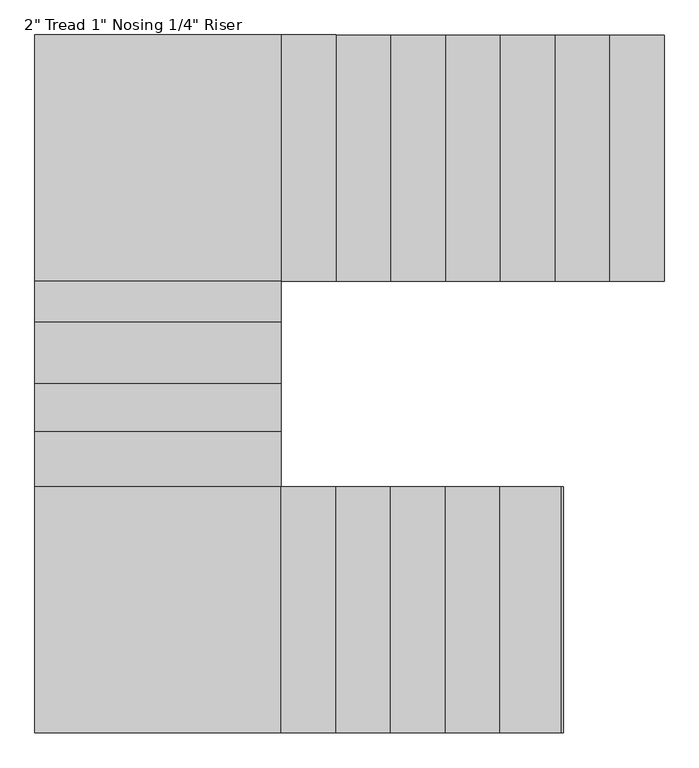
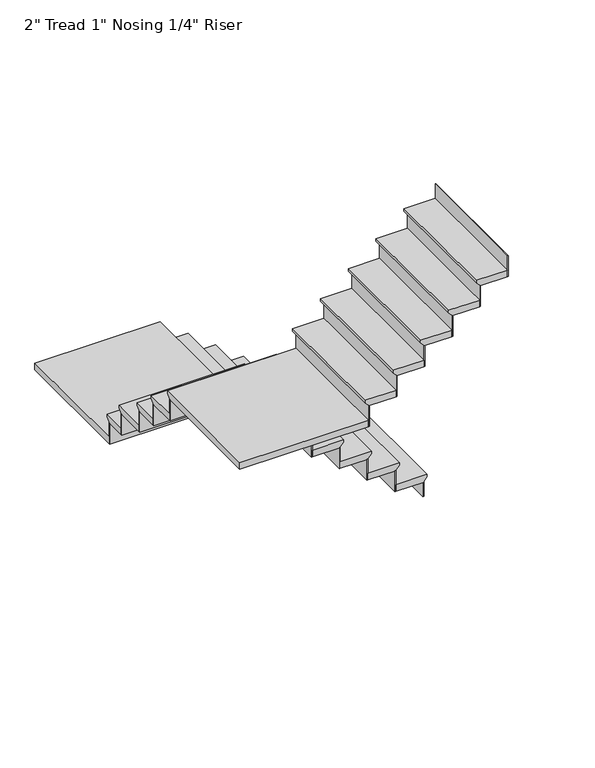
"""IFC4 building model written with IfcOpenShell, lengths in millimetres: stair flight geometry."""

from ifc_helpers import new_model, si_unit, origin, place, context, project, spatial, faceted_brep, source, transform, mapped, element, save


def stair_flight_03a67781(model_context):
    return source(origin(), model_context, "Body", "Brep", [
        faceted_brep([(-3603.1340247, 922.0319954, 9742.5710526), (-3603.1340247, 922.0319954, 9761.6210526), (-3603.1340247, 7.6319954, 9761.6210526), (-3603.1340247, 7.6319954, 9742.5710526), (-3628.5340247, 922.0319954, 9717.1710526), (-3628.5340247, 7.6319954, 9717.1710526), (-3831.7340247, 922.0319954, 9761.6210526), (-3831.7340247, 7.6319954, 9761.6210526), (-3628.5340247, 7.6319954, 9710.8210526), (-3831.7340247, 7.6319954, 9710.8210526), (-3831.7340247, 922.0319954, 9710.8210526), (-3628.5340247, 922.0319954, 9710.8210526)], [[[0, 1, 2, 3]], [[4, 0, 3, 5]], [[2, 1, 6, 7]], [[8, 9, 10, 11]], [[2, 7, 9, 8, 5, 3]], [[8, 11, 4, 5]], [[6, 1, 0, 4, 11, 10]], [[7, 6, 10, 9]]]),
        faceted_brep([(-3628.5340247, 922.0319954, 9710.8210526), (-3628.5340247, 922.0319954, 9601.2), (-3634.8840247, 922.0319954, 9601.2), (-3634.8840247, 922.0319954, 9710.8210526), (-3628.5340247, 7.6319954, 9710.8210526), (-3634.8840247, 7.6319954, 9710.8210526), (-3634.8840247, 7.6319954, 9601.2), (-3628.5340247, 7.6319954, 9601.2)], [[[0, 1, 2, 3]], [[4, 5, 6, 7]], [[1, 0, 4, 7]], [[2, 1, 7, 6]], [[3, 2, 6, 5]], [[0, 3, 5, 4]]]),
        faceted_brep([(-3831.7340247, 922.0319954, 9871.2421053), (-3831.7340247, 922.0319954, 9710.8210526), (-3838.0840247, 922.0319954, 9710.8210526), (-3838.0840247, 922.0319954, 9871.2421053), (-3831.7340247, 7.6319954, 9871.2421053), (-3838.0840247, 7.6319954, 9871.2421053), (-3838.0840247, 7.6319954, 9710.8210526), (-3831.7340247, 7.6319954, 9710.8210526)], [[[0, 1, 2, 3]], [[4, 5, 6, 7]], [[1, 0, 4, 7]], [[2, 1, 7, 6]], [[3, 2, 6, 5]], [[0, 3, 5, 4]]]),
        faceted_brep([(-3806.3340247, 7.6319954, 9922.0421053), (-3806.3340247, 922.0319954, 9922.0421053), (-4034.9340247, 922.0319954, 9922.0421053), (-4034.9340247, 7.6319954, 9922.0421053), (-3831.7340247, 7.6319954, 9871.2421053), (-4034.9340247, 7.6319954, 9871.2421053), (-4034.9340247, 922.0319954, 9871.2421053), (-3831.7340247, 922.0319954, 9871.2421053), (-3831.7340247, 7.6319954, 9877.5921053), (-3806.3340247, 7.6319954, 9902.9921053), (-3831.7340247, 922.0319954, 9877.5921053), (-3806.3340247, 922.0319954, 9902.9921053)], [[[0, 1, 2, 3]], [[4, 5, 6, 7]], [[0, 3, 5, 4, 8, 9]], [[4, 7, 10, 8]], [[2, 1, 11, 10, 7, 6]], [[3, 2, 6, 5]], [[11, 1, 0, 9]], [[10, 11, 9, 8]]]),
        faceted_brep([(-4034.9340247, 922.0319954, 10031.6631579), (-4034.9340247, 922.0319954, 9871.2421053), (-4041.2840247, 922.0319954, 9871.2421053), (-4041.2840247, 922.0319954, 10031.6631579), (-4034.9340247, 7.6319954, 10031.6631579), (-4041.2840247, 7.6319954, 10031.6631579), (-4041.2840247, 7.6319954, 9871.2421053), (-4034.9340247, 7.6319954, 9871.2421053)], [[[0, 1, 2, 3]], [[4, 5, 6, 7]], [[1, 0, 4, 7]], [[2, 1, 7, 6]], [[3, 2, 6, 5]], [[0, 3, 5, 4]]]),
        faceted_brep([(-4009.5340247, 7.6319954, 10082.4631579), (-4009.5340247, 922.0319954, 10082.4631579), (-4238.1340247, 922.0319954, 10082.4631579), (-4238.1340247, 7.6319954, 10082.4631579), (-4034.9340247, 7.6319954, 10031.6631579), (-4238.1340247, 7.6319954, 10031.6631579), (-4238.1340247, 922.0319954, 10031.6631579), (-4034.9340247, 922.0319954, 10031.6631579), (-4034.9340247, 7.6319954, 10038.0131579), (-4009.5340247, 7.6319954, 10063.4131579), (-4034.9340247, 922.0319954, 10038.0131579), (-4009.5340247, 922.0319954, 10063.4131579)], [[[0, 1, 2, 3]], [[4, 5, 6, 7]], [[0, 3, 5, 4, 8, 9]], [[4, 7, 10, 8]], [[2, 1, 11, 10, 7, 6]], [[3, 2, 6, 5]], [[11, 1, 0, 9]], [[10, 11, 9, 8]]]),
        faceted_brep([(-4238.1340247, 922.0319954, 10192.0842105), (-4238.1340247, 922.0319954, 10031.6631579), (-4244.4840247, 922.0319954, 10031.6631579), (-4244.4840247, 922.0319954, 10192.0842105), (-4238.1340247, 7.6319954, 10192.0842105), (-4244.4840247, 7.6319954, 10192.0842105), (-4244.4840247, 7.6319954, 10031.6631579), (-4238.1340247, 7.6319954, 10031.6631579)], [[[0, 1, 2, 3]], [[4, 5, 6, 7]], [[1, 0, 4, 7]], [[2, 1, 7, 6]], [[3, 2, 6, 5]], [[0, 3, 5, 4]]]),
        faceted_brep([(-4212.7340247, 7.6319954, 10242.8842105), (-4212.7340247, 922.0319954, 10242.8842105), (-4441.3340247, 922.0319954, 10242.8842105), (-4441.3340247, 7.6319954, 10242.8842105), (-4238.1340247, 7.6319954, 10192.0842105), (-4441.3340247, 7.6319954, 10192.0842105), (-4441.3340247, 922.0319954, 10192.0842105), (-4238.1340247, 922.0319954, 10192.0842105), (-4238.1340247, 7.6319954, 10198.4342105), (-4212.7340247, 7.6319954, 10223.8342105), (-4238.1340247, 922.0319954, 10198.4342105), (-4212.7340247, 922.0319954, 10223.8342105)], [[[0, 1, 2, 3]], [[4, 5, 6, 7]], [[0, 3, 5, 4, 8, 9]], [[4, 7, 10, 8]], [[2, 1, 11, 10, 7, 6]], [[3, 2, 6, 5]], [[11, 1, 0, 9]], [[10, 11, 9, 8]]]),
        faceted_brep([(-4441.3340247, 922.0319954, 10352.5052632), (-4441.3340247, 922.0319954, 10192.0842105), (-4447.6840247, 922.0319954, 10192.0842105), (-4447.6840247, 922.0319954, 10352.5052632), (-4441.3340247, 7.6319954, 10352.5052632), (-4447.6840247, 7.6319954, 10352.5052632), (-4447.6840247, 7.6319954, 10192.0842105), (-4441.3340247, 7.6319954, 10192.0842105)], [[[0, 1, 2, 3]], [[4, 5, 6, 7]], [[1, 0, 4, 7]], [[2, 1, 7, 6]], [[3, 2, 6, 5]], [[0, 3, 5, 4]]]),
        faceted_brep([(-4415.9340247, 7.6319954, 10403.3052632), (-4415.9340247, 922.0319954, 10403.3052632), (-4644.5340247, 922.0319954, 10403.3052632), (-4644.5340247, 7.6319954, 10403.3052632), (-4441.3340247, 7.6319954, 10352.5052632), (-4644.5340247, 7.6319954, 10352.5052632), (-4644.5340247, 922.0319954, 10352.5052632), (-4441.3340247, 922.0319954, 10352.5052632), (-4441.3340247, 7.6319954, 10358.8552632), (-4415.9340247, 7.6319954, 10384.2552632), (-4441.3340247, 922.0319954, 10358.8552632), (-4415.9340247, 922.0319954, 10384.2552632)], [[[0, 1, 2, 3]], [[4, 5, 6, 7]], [[0, 3, 5, 4, 8, 9]], [[4, 7, 10, 8]], [[2, 1, 11, 10, 7, 6]], [[3, 2, 6, 5]], [[11, 1, 0, 9]], [[10, 11, 9, 8]]]),
        faceted_brep([(-4644.5340247, 922.0319954, 10512.9263158), (-4644.5340247, 922.0319954, 10352.5052632), (-4650.8840247, 922.0319954, 10352.5052632), (-4650.8840247, 922.0319954, 10512.9263158), (-4644.5340247, 7.6319954, 10512.9263158), (-4650.8840247, 7.6319954, 10512.9263158), (-4650.8840247, 7.6319954, 10352.5052632), (-4644.5340247, 7.6319954, 10352.5052632)], [[[0, 1, 2, 3]], [[4, 5, 6, 7]], [[1, 0, 4, 7]], [[2, 1, 7, 6]], [[3, 2, 6, 5]], [[0, 3, 5, 4]]]),
        faceted_brep([(-4619.1340247, 7.6319954, 10563.7263158), (-4619.1340247, 922.0319954, 10563.7263158), (-4847.7340247, 922.0319954, 10563.7263158), (-4847.7340247, 7.6319954, 10563.7263158), (-4644.5340247, 7.6319954, 10512.9263158), (-4847.7340247, 7.6319954, 10512.9263158), (-4847.7340247, 922.0319954, 10512.9263158), (-4644.5340247, 922.0319954, 10512.9263158), (-4644.5340247, 7.6319954, 10519.2763158), (-4619.1340247, 7.6319954, 10544.6763158), (-4644.5340247, 922.0319954, 10519.2763158), (-4619.1340247, 922.0319954, 10544.6763158)], [[[0, 1, 2, 3]], [[4, 5, 6, 7]], [[0, 3, 5, 4, 8, 9]], [[4, 7, 10, 8]], [[2, 1, 11, 10, 7, 6]], [[3, 2, 6, 5]], [[11, 1, 0, 9]], [[10, 11, 9, 8]]]),
        faceted_brep([(-4847.7340247, 922.0319954, 10673.3473684), (-4847.7340247, 922.0319954, 10512.9263158), (-4854.0840247, 922.0319954, 10512.9263158), (-4854.0840247, 922.0319954, 10673.3473684), (-4847.7340247, 7.6319954, 10673.3473684), (-4854.0840247, 7.6319954, 10673.3473684), (-4854.0840247, 7.6319954, 10512.9263158), (-4847.7340247, 7.6319954, 10512.9263158)], [[[0, 1, 2, 3]], [[4, 5, 6, 7]], [[1, 0, 4, 7]], [[2, 1, 7, 6]], [[3, 2, 6, 5]], [[0, 3, 5, 4]]]),
        faceted_brep([(-4822.3340247, 7.6319954, 10724.1473684), (-4822.3340247, 922.0319954, 10724.1473684), (-5050.9340247, 922.0319954, 10724.1473684), (-5050.9340247, 7.6319954, 10724.1473684), (-4847.7340247, 7.6319954, 10673.3473684), (-5050.9340247, 7.6319954, 10673.3473684), (-5050.9340247, 922.0319954, 10673.3473684), (-4847.7340247, 922.0319954, 10673.3473684), (-4847.7340247, 7.6319954, 10679.6973684), (-4822.3340247, 7.6319954, 10705.0973684), (-4847.7340247, 922.0319954, 10679.6973684), (-4822.3340247, 922.0319954, 10705.0973684)], [[[0, 1, 2, 3]], [[4, 5, 6, 7]], [[0, 3, 5, 4, 8, 9]], [[4, 7, 10, 8]], [[2, 1, 11, 10, 7, 6]], [[3, 2, 6, 5]], [[11, 1, 0, 9]], [[10, 11, 9, 8]]]),
        faceted_brep([(-5050.9340247, 922.0319954, 10833.7684211), (-5050.9340247, 922.0319954, 10673.3473684), (-5057.2840247, 922.0319954, 10673.3473684), (-5057.2840247, 922.0319954, 10833.7684211), (-5050.9340247, 7.6319954, 10833.7684211), (-5057.2840247, 7.6319954, 10833.7684211), (-5057.2840247, 7.6319954, 10673.3473684), (-5050.9340247, 7.6319954, 10673.3473684)], [[[0, 1, 2, 3]], [[4, 5, 6, 7]], [[1, 0, 4, 7]], [[2, 1, 7, 6]], [[3, 2, 6, 5]], [[0, 3, 5, 4]]]),
        faceted_brep([(-5939.9340247, 922.0319954, 10884.5684211), (-5939.9340247, -17.7680046, 10884.5684211), (-5025.5340247, -17.7680046, 10884.5684211), (-5025.5340247, 922.0319954, 10884.5684211), (-5025.5340247, 7.6319954, 10833.7684211), (-5025.5340247, -17.7680046, 10833.7684211), (-5939.9340247, -17.7680046, 10833.7684211), (-5939.9340247, 922.0319954, 10833.7684211), (-5050.9340247, 922.0319954, 10833.7684211), (-5050.9340247, 7.6319954, 10833.7684211), (-5025.5340247, 7.6319954, 10865.5184211), (-5025.5340247, 922.0319954, 10865.5184211), (-5050.9340247, 7.6319954, 10840.1184211), (-5050.9340247, 922.0319954, 10840.1184211)], [[[0, 1, 2, 3]], [[4, 5, 6, 7, 8, 9]], [[3, 2, 5, 4, 10, 11]], [[4, 9, 12, 10]], [[9, 8, 13, 12]], [[0, 3, 11, 13, 8, 7]], [[1, 0, 7, 6]], [[2, 1, 6, 5]], [[13, 11, 10, 12]]]),
        faceted_brep([(-5939.9340247, -17.7680046, 10994.1894737), (-5939.9340247, -17.7680046, 10833.7684211), (-5939.9340247, -24.1180046, 10833.7684211), (-5939.9340247, -24.1180046, 10994.1894737), (-5025.5340247, -17.7680046, 10994.1894737), (-5025.5340247, -24.1180046, 10994.1894737), (-5025.5340247, -24.1180046, 10833.7684211), (-5025.5340247, -17.7680046, 10833.7684211)], [[[0, 1, 2, 3]], [[4, 5, 6, 7]], [[1, 0, 4, 7]], [[2, 1, 7, 6]], [[3, 2, 6, 5]], [[0, 3, 5, 4]]]),
        faceted_brep([(-5025.5340247, 7.6319954, 11044.9894737), (-5939.9340247, 7.6319954, 11044.9894737), (-5939.9340247, -170.1680046, 11044.9894737), (-5025.5340247, -170.1680046, 11044.9894737), (-5025.5340247, -17.7680046, 10994.1894737), (-5025.5340247, -170.1680046, 10994.1894737), (-5939.9340247, -170.1680046, 10994.1894737), (-5939.9340247, -17.7680046, 10994.1894737), (-5025.5340247, -17.7680046, 11000.5394737), (-5025.5340247, 7.6319954, 11025.9394737), (-5939.9340247, -17.7680046, 11000.5394737), (-5939.9340247, 7.6319954, 11025.9394737)], [[[0, 1, 2, 3]], [[4, 5, 6, 7]], [[0, 3, 5, 4, 8, 9]], [[4, 7, 10, 8]], [[2, 1, 11, 10, 7, 6]], [[3, 2, 6, 5]], [[11, 1, 0, 9]], [[10, 11, 9, 8]]]),
        faceted_brep([(-5939.9340247, -170.1680046, 11154.6105263), (-5939.9340247, -170.1680046, 10994.1894737), (-5939.9340247, -176.5180046, 10994.1894737), (-5939.9340247, -176.5180046, 11154.6105263), (-5025.5340247, -170.1680046, 11154.6105263), (-5025.5340247, -176.5180046, 11154.6105263), (-5025.5340247, -176.5180046, 10994.1894737), (-5025.5340247, -170.1680046, 10994.1894737)], [[[0, 1, 2, 3]], [[4, 5, 6, 7]], [[1, 0, 4, 7]], [[2, 1, 7, 6]], [[3, 2, 6, 5]], [[0, 3, 5, 4]]]),
        faceted_brep([(-5025.5340247, -144.7680046, 11205.4105263), (-5939.9340247, -144.7680046, 11205.4105263), (-5939.9340247, -398.7680046, 11205.4105263), (-5025.5340247, -398.7680046, 11205.4105263), (-5025.5340247, -170.1680046, 11154.6105263), (-5025.5340247, -398.7680046, 11154.6105263), (-5939.9340247, -398.7680046, 11154.6105263), (-5939.9340247, -170.1680046, 11154.6105263), (-5025.5340247, -170.1680046, 11160.9605263), (-5025.5340247, -144.7680046, 11186.3605263), (-5939.9340247, -170.1680046, 11160.9605263), (-5939.9340247, -144.7680046, 11186.3605263)], [[[0, 1, 2, 3]], [[4, 5, 6, 7]], [[0, 3, 5, 4, 8, 9]], [[4, 7, 10, 8]], [[2, 1, 11, 10, 7, 6]], [[3, 2, 6, 5]], [[11, 1, 0, 9]], [[10, 11, 9, 8]]]),
        faceted_brep([(-5939.9340247, -398.7680046, 11315.0315789), (-5939.9340247, -398.7680046, 11154.6105263), (-5939.9340247, -405.1180046, 11154.6105263), (-5939.9340247, -405.1180046, 11315.0315789), (-5025.5340247, -398.7680046, 11315.0315789), (-5025.5340247, -405.1180046, 11315.0315789), (-5025.5340247, -405.1180046, 11154.6105263), (-5025.5340247, -398.7680046, 11154.6105263)], [[[0, 1, 2, 3]], [[4, 5, 6, 7]], [[1, 0, 4, 7]], [[2, 1, 7, 6]], [[3, 2, 6, 5]], [[0, 3, 5, 4]]]),
        faceted_brep([(-5025.5340247, -373.3680046, 11365.8315789), (-5939.9340247, -373.3680046, 11365.8315789), (-5939.9340247, -576.5680046, 11365.8315789), (-5025.5340247, -576.5680046, 11365.8315789), (-5025.5340247, -398.7680046, 11315.0315789), (-5025.5340247, -576.5680046, 11315.0315789), (-5939.9340247, -576.5680046, 11315.0315789), (-5939.9340247, -398.7680046, 11315.0315789), (-5025.5340247, -398.7680046, 11321.3815789), (-5025.5340247, -373.3680046, 11346.7815789), (-5939.9340247, -398.7680046, 11321.3815789), (-5939.9340247, -373.3680046, 11346.7815789)], [[[0, 1, 2, 3]], [[4, 5, 6, 7]], [[0, 3, 5, 4, 8, 9]], [[4, 7, 10, 8]], [[2, 1, 11, 10, 7, 6]], [[3, 2, 6, 5]], [[11, 1, 0, 9]], [[10, 11, 9, 8]]]),
        faceted_brep([(-5939.9340247, -576.5680046, 11475.4526316), (-5939.9340247, -576.5680046, 11315.0315789), (-5939.9340247, -582.9180046, 11315.0315789), (-5939.9340247, -582.9180046, 11475.4526316), (-5025.5340247, -576.5680046, 11475.4526316), (-5025.5340247, -582.9180046, 11475.4526316), (-5025.5340247, -582.9180046, 11315.0315789), (-5025.5340247, -576.5680046, 11315.0315789)], [[[0, 1, 2, 3]], [[4, 5, 6, 7]], [[1, 0, 4, 7]], [[2, 1, 7, 6]], [[3, 2, 6, 5]], [[0, 3, 5, 4]]]),
        faceted_brep([(-5025.5340247, -551.1680046, 11526.2526316), (-5939.9340247, -551.1680046, 11526.2526316), (-5939.9340247, -779.7680046, 11526.2526316), (-5025.5340247, -779.7680046, 11526.2526316), (-5025.5340247, -576.5680046, 11475.4526316), (-5025.5340247, -779.7680046, 11475.4526316), (-5939.9340247, -779.7680046, 11475.4526316), (-5939.9340247, -576.5680046, 11475.4526316), (-5025.5340247, -576.5680046, 11481.8026316), (-5025.5340247, -551.1680046, 11507.2026316), (-5939.9340247, -576.5680046, 11481.8026316), (-5939.9340247, -551.1680046, 11507.2026316)], [[[0, 1, 2, 3]], [[4, 5, 6, 7]], [[0, 3, 5, 4, 8, 9]], [[4, 7, 10, 8]], [[2, 1, 11, 10, 7, 6]], [[3, 2, 6, 5]], [[11, 1, 0, 9]], [[10, 11, 9, 8]]]),
        faceted_brep([(-5939.9340247, -779.7680046, 11635.8736842), (-5939.9340247, -779.7680046, 11475.4526316), (-5939.9340247, -786.1180046, 11475.4526316), (-5939.9340247, -786.1180046, 11635.8736842), (-5025.5340247, -779.7680046, 11635.8736842), (-5025.5340247, -786.1180046, 11635.8736842), (-5025.5340247, -786.1180046, 11475.4526316), (-5025.5340247, -779.7680046, 11475.4526316)], [[[0, 1, 2, 3]], [[4, 5, 6, 7]], [[1, 0, 4, 7]], [[2, 1, 7, 6]], [[3, 2, 6, 5]], [[0, 3, 5, 4]]]),
        faceted_brep([(-5939.9340247, -1668.7680046, 11686.6736842), (-5000.1340247, -1668.7680046, 11686.6736842), (-5000.1340247, -754.3680046, 11686.6736842), (-5939.9340247, -754.3680046, 11686.6736842), (-5025.5340247, -754.3680046, 11635.8736842), (-5000.1340247, -754.3680046, 11635.8736842), (-5000.1340247, -1668.7680046, 11635.8736842), (-5939.9340247, -1668.7680046, 11635.8736842), (-5939.9340247, -779.7680046, 11635.8736842), (-5025.5340247, -779.7680046, 11635.8736842), (-5025.5340247, -754.3680046, 11667.6236842), (-5939.9340247, -754.3680046, 11667.6236842), (-5025.5340247, -779.7680046, 11642.2236842), (-5939.9340247, -779.7680046, 11642.2236842)], [[[0, 1, 2, 3]], [[4, 5, 6, 7, 8, 9]], [[3, 2, 5, 4, 10, 11]], [[4, 9, 12, 10]], [[9, 8, 13, 12]], [[0, 3, 11, 13, 8, 7]], [[1, 0, 7, 6]], [[2, 1, 6, 5]], [[13, 11, 10, 12]]]),
        faceted_brep([(-5000.1340247, -1668.7680046, 11796.2947368), (-5000.1340247, -1668.7680046, 11635.8736842), (-4993.7840247, -1668.7680046, 11635.8736842), (-4993.7840247, -1668.7680046, 11796.2947368), (-5000.1340247, -754.3680046, 11796.2947368), (-4993.7840247, -754.3680046, 11796.2947368), (-4993.7840247, -754.3680046, 11635.8736842), (-5000.1340247, -754.3680046, 11635.8736842)], [[[0, 1, 2, 3]], [[4, 5, 6, 7]], [[1, 0, 4, 7]], [[2, 1, 7, 6]], [[3, 2, 6, 5]], [[0, 3, 5, 4]]]),
        faceted_brep([(-5025.5340247, -754.3680046, 11847.0947368), (-5025.5340247, -1668.7680046, 11847.0947368), (-4796.9340247, -1668.7680046, 11847.0947368), (-4796.9340247, -754.3680046, 11847.0947368), (-5000.1340247, -754.3680046, 11796.2947368), (-4796.9340247, -754.3680046, 11796.2947368), (-4796.9340247, -1668.7680046, 11796.2947368), (-5000.1340247, -1668.7680046, 11796.2947368), (-5000.1340247, -754.3680046, 11802.6447368), (-5025.5340247, -754.3680046, 11828.0447368), (-5000.1340247, -1668.7680046, 11802.6447368), (-5025.5340247, -1668.7680046, 11828.0447368)], [[[0, 1, 2, 3]], [[4, 5, 6, 7]], [[0, 3, 5, 4, 8, 9]], [[4, 7, 10, 8]], [[2, 1, 11, 10, 7, 6]], [[3, 2, 6, 5]], [[11, 1, 0, 9]], [[10, 11, 9, 8]]]),
        faceted_brep([(-4796.9340247, -1668.7680046, 11956.7157895), (-4796.9340247, -1668.7680046, 11796.2947368), (-4790.5840247, -1668.7680046, 11796.2947368), (-4790.5840247, -1668.7680046, 11956.7157895), (-4796.9340247, -754.3680046, 11956.7157895), (-4790.5840247, -754.3680046, 11956.7157895), (-4790.5840247, -754.3680046, 11796.2947368), (-4796.9340247, -754.3680046, 11796.2947368)], [[[0, 1, 2, 3]], [[4, 5, 6, 7]], [[1, 0, 4, 7]], [[2, 1, 7, 6]], [[3, 2, 6, 5]], [[0, 3, 5, 4]]]),
        faceted_brep([(-4822.3340247, -754.3680046, 12007.5157895), (-4822.3340247, -1668.7680046, 12007.5157895), (-4593.7340247, -1668.7680046, 12007.5157895), (-4593.7340247, -754.3680046, 12007.5157895), (-4796.9340247, -754.3680046, 11956.7157895), (-4593.7340247, -754.3680046, 11956.7157895), (-4593.7340247, -1668.7680046, 11956.7157895), (-4796.9340247, -1668.7680046, 11956.7157895), (-4796.9340247, -754.3680046, 11963.0657895), (-4822.3340247, -754.3680046, 11988.4657895), (-4796.9340247, -1668.7680046, 11963.0657895), (-4822.3340247, -1668.7680046, 11988.4657895)], [[[0, 1, 2, 3]], [[4, 5, 6, 7]], [[0, 3, 5, 4, 8, 9]], [[4, 7, 10, 8]], [[2, 1, 11, 10, 7, 6]], [[3, 2, 6, 5]], [[11, 1, 0, 9]], [[10, 11, 9, 8]]]),
        faceted_brep([(-4593.7340247, -1668.7680046, 12117.1368421), (-4593.7340247, -1668.7680046, 11956.7157895), (-4587.3840247, -1668.7680046, 11956.7157895), (-4587.3840247, -1668.7680046, 12117.1368421), (-4593.7340247, -754.3680046, 12117.1368421), (-4587.3840247, -754.3680046, 12117.1368421), (-4587.3840247, -754.3680046, 11956.7157895), (-4593.7340247, -754.3680046, 11956.7157895)], [[[0, 1, 2, 3]], [[4, 5, 6, 7]], [[1, 0, 4, 7]], [[2, 1, 7, 6]], [[3, 2, 6, 5]], [[0, 3, 5, 4]]]),
        faceted_brep([(-4619.1340247, -754.3680046, 12167.9368421), (-4619.1340247, -1668.7680046, 12167.9368421), (-4390.5340247, -1668.7680046, 12167.9368421), (-4390.5340247, -754.3680046, 12167.9368421), (-4593.7340247, -754.3680046, 12117.1368421), (-4390.5340247, -754.3680046, 12117.1368421), (-4390.5340247, -1668.7680046, 12117.1368421), (-4593.7340247, -1668.7680046, 12117.1368421), (-4593.7340247, -754.3680046, 12123.4868421), (-4619.1340247, -754.3680046, 12148.8868421), (-4593.7340247, -1668.7680046, 12123.4868421), (-4619.1340247, -1668.7680046, 12148.8868421)], [[[0, 1, 2, 3]], [[4, 5, 6, 7]], [[0, 3, 5, 4, 8, 9]], [[4, 7, 10, 8]], [[2, 1, 11, 10, 7, 6]], [[3, 2, 6, 5]], [[11, 1, 0, 9]], [[10, 11, 9, 8]]]),
        faceted_brep([(-4390.5340247, -1668.7680046, 12277.5578947), (-4390.5340247, -1668.7680046, 12117.1368421), (-4384.1840247, -1668.7680046, 12117.1368421), (-4384.1840247, -1668.7680046, 12277.5578947), (-4390.5340247, -754.3680046, 12277.5578947), (-4384.1840247, -754.3680046, 12277.5578947), (-4384.1840247, -754.3680046, 12117.1368421), (-4390.5340247, -754.3680046, 12117.1368421)], [[[0, 1, 2, 3]], [[4, 5, 6, 7]], [[1, 0, 4, 7]], [[2, 1, 7, 6]], [[3, 2, 6, 5]], [[0, 3, 5, 4]]]),
        faceted_brep([(-4415.9340247, -754.3680046, 12328.3578947), (-4415.9340247, -1668.7680046, 12328.3578947), (-4187.3340247, -1668.7680046, 12328.3578947), (-4187.3340247, -754.3680046, 12328.3578947), (-4390.5340247, -754.3680046, 12277.5578947), (-4187.3340247, -754.3680046, 12277.5578947), (-4187.3340247, -1668.7680046, 12277.5578947), (-4390.5340247, -1668.7680046, 12277.5578947), (-4390.5340247, -754.3680046, 12283.9078947), (-4415.9340247, -754.3680046, 12309.3078947), (-4390.5340247, -1668.7680046, 12283.9078947), (-4415.9340247, -1668.7680046, 12309.3078947)], [[[0, 1, 2, 3]], [[4, 5, 6, 7]], [[0, 3, 5, 4, 8, 9]], [[4, 7, 10, 8]], [[2, 1, 11, 10, 7, 6]], [[3, 2, 6, 5]], [[11, 1, 0, 9]], [[10, 11, 9, 8]]]),
        faceted_brep([(-4187.3340247, -1668.7680046, 12437.9789474), (-4187.3340247, -1668.7680046, 12277.5578947), (-4180.9840247, -1668.7680046, 12277.5578947), (-4180.9840247, -1668.7680046, 12437.9789474), (-4187.3340247, -754.3680046, 12437.9789474), (-4180.9840247, -754.3680046, 12437.9789474), (-4180.9840247, -754.3680046, 12277.5578947), (-4187.3340247, -754.3680046, 12277.5578947)], [[[0, 1, 2, 3]], [[4, 5, 6, 7]], [[1, 0, 4, 7]], [[2, 1, 7, 6]], [[3, 2, 6, 5]], [[0, 3, 5, 4]]]),
        faceted_brep([(-3984.1340247, -1668.7680046, 12598.4), (-3984.1340247, -1668.7680046, 12437.9789474), (-3977.7840247, -1668.7680046, 12437.9789474), (-3977.7840247, -1668.7680046, 12598.4), (-3984.1340247, -754.3680046, 12598.4), (-3977.7840247, -754.3680046, 12598.4), (-3977.7840247, -754.3680046, 12437.9789474), (-3984.1340247, -754.3680046, 12437.9789474)], [[[0, 1, 2, 3]], [[4, 5, 6, 7]], [[1, 0, 4, 7]], [[2, 1, 7, 6]], [[3, 2, 6, 5]], [[0, 3, 5, 4]]]),
        faceted_brep([(-4212.7340247, -754.3680046, 12488.7789474), (-4212.7340247, -1668.7680046, 12488.7789474), (-3984.1340247, -1668.7680046, 12488.7789474), (-3984.1340247, -754.3680046, 12488.7789474), (-4187.3340247, -754.3680046, 12437.9789474), (-3984.1340247, -754.3680046, 12437.9789474), (-3984.1340247, -1668.7680046, 12437.9789474), (-4187.3340247, -1668.7680046, 12437.9789474), (-4187.3340247, -754.3680046, 12444.3289474), (-4212.7340247, -754.3680046, 12469.7289474), (-4187.3340247, -1668.7680046, 12444.3289474), (-4212.7340247, -1668.7680046, 12469.7289474)], [[[0, 1, 2, 3]], [[4, 5, 6, 7]], [[0, 3, 5, 4, 8, 9]], [[4, 7, 10, 8]], [[2, 1, 11, 10, 7, 6]], [[3, 2, 6, 5]], [[11, 1, 0, 9]], [[10, 11, 9, 8]]]),
    ])


if __name__ == "__main__":
    model = new_model("IFC4")
    model_context = context("Model", 3, world=origin())
    ifc_project = project(units=[si_unit("LENGTHUNIT", "METRE", prefix="MILLI")], contexts=[model_context])
    site = spatial("IfcSite", under=ifc_project)
    building = spatial("IfcBuilding", under=site)
    placement = place(None, origin())
    stair_flight_shape = stair_flight_03a67781(model_context)
    element("IfcStairFlight", 1, ObjectType="2\" Tread 1\" Nosing 1/4\" Riser", at=placement, inside=building, context=model_context, shape_type="MappedRepresentation", body=[
        mapped(stair_flight_shape, transform((0.0, 0.0, 0.0), x_axis=(1.0, 0.0, 0.0), y_axis=(0.0, 1.0, 0.0), z_axis=(0.0, 0.0, 1.0))),
    ])
    save(model, "model.ifc")
